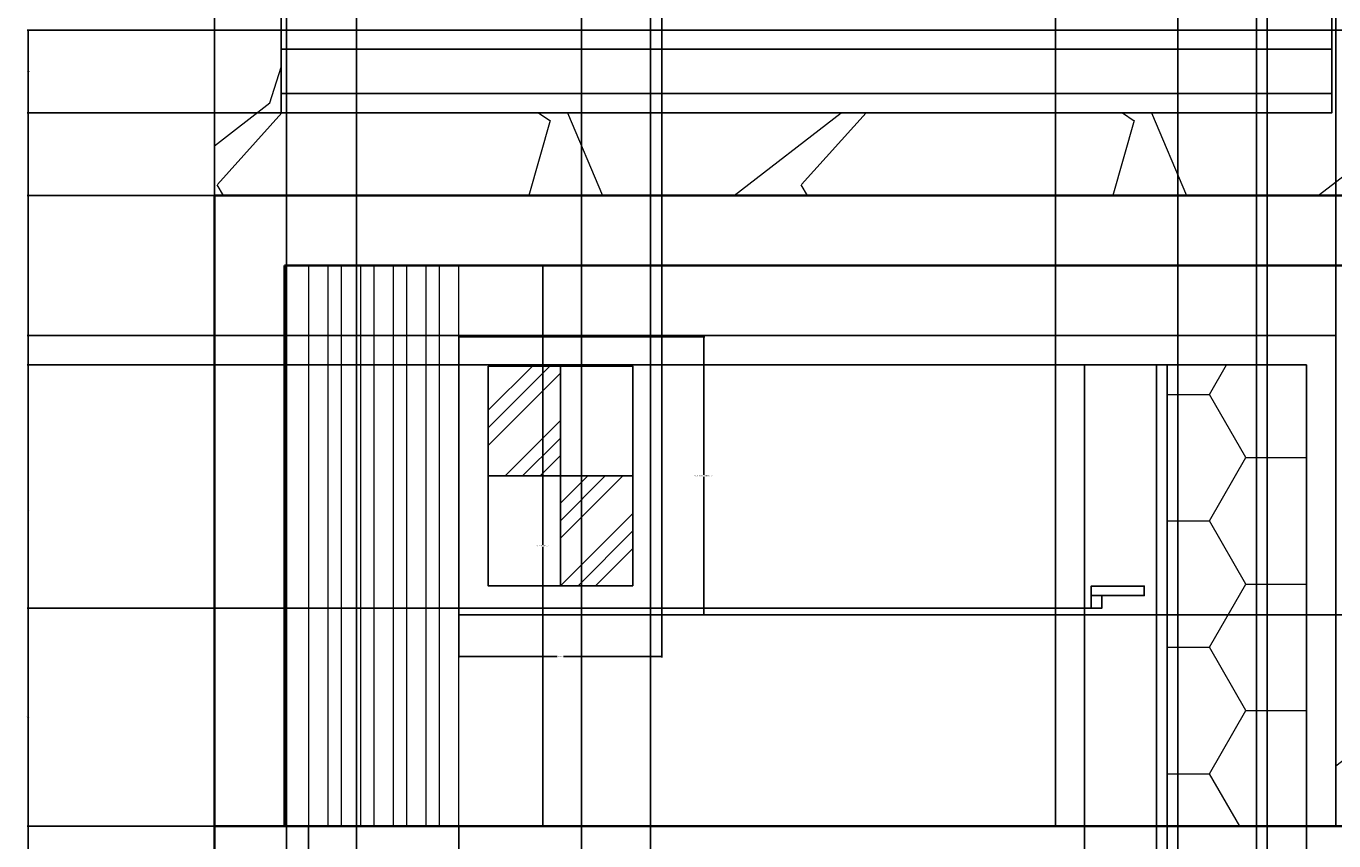
# Model space of a CAD drawing. Units: inches. Extents: x -8 to 554, y -200 to 499.
# Tile 7 of 12: x -8 to 216, y 233 to 372. Entities that reach past the tile are written whole.
import ezdxf

# ---------------------------------------------------------------- set-up
doc = ezdxf.new("R2010")
doc.units = ezdxf.units.IN
doc.header["$MEASUREMENT"] = 0
for name, color, linetype, lineweight in [('A-ANNO-DIMS', 2, 'Continuous', 18), ('A-DOOR', 3, 'Continuous', 25), ('A-DOOR-PATT', 252, 'Continuous', 13), ('A-FLOR', 7, 'Continuous', 35), ('A-GLAZ', 4, 'Continuous', 25), ('A-GLAZ-PATT', 252, 'Continuous', 13), ('A-WALL', 7, 'Continuous', 35), ('A-WALL-PATT', 252, 'Continuous', 13), ('A-WALL-PRPT', 7, 'Continuous', 25), ('A-WALL-SCRN', 8, 'Continuous', 18)]:
    doc.layers.add(name, color=color, linetype=linetype, lineweight=lineweight)
doc.styles.get("Standard").update_dxf_attribs({"font": 'arial.ttf'})
doc.dimstyles.get("Standard").update_dxf_attribs({"dimtxt": 0.18, "dimasz": 0.18, "dimexe": 0.18, "dimexo": 0.0625, "dimgap": 0.09, "dimtad": 0, "dimtih": 1, "dimtoh": 1, "dimdec": 4, "dimzin": 0, "dimdsep": 46, "dimtxsty": 'Standard', "dimcen": 0.09, "dimadec": 0, "dimazin": 0, "dimtfac": 1, "dimtdec": 4, "dimtofl": 0, "dimtmove": 0, "dimatfit": 3, "dimfxl": 1, "dimtolj": 1, "dimtzin": 0, "dimarcsym": 0})

# ---------------------------------------------------------------- blocks, each defined once
blk = doc.blocks.new('DOOR-LEVER-ELEV')
for points in [[(0, 2.19), (9.08, 2.19), (9.08, 3.81), (0, 3.81)], [(0, 2.19), (1.8, 2.19), (1.8, 0), (0, 0)]]:
    blk.add_lwpolyline(points, close=True)
blk = doc.blocks.new('SCREEN-FIVE-FINS-ELEV')
for points in [[(0, 0), (3.37, 0), (3.37, 96), (0, 96)], [(5.59, 0), (8.97, 0), (8.97, 96), (5.59, 96)], [(11.19, 0), (14.56, 0), (14.56, 96), (11.19, 96)], [(16.78, 0), (20.16, 0), (20.16, 96), (16.78, 96)], [(22.38, 0), (25.75, 0), (25.75, 96), (22.38, 96)]]:
    blk.add_lwpolyline(points, close=True)
blk = doc.blocks.new('WINDOW-CASING-FOUR-LIGHT')
blk.add_lwpolyline([(0, 47.61), (34.77, 47.61), (34.77, 0), (0, 0)], close=True)
blk = doc.blocks.new('*D18')
at = {"layer": 'A-ANNO-DIMS', "color": 0, "lineweight": -2, "transparency": 16777216}
for p, q in [((66.27, 331.48), (80.78, 331.48)), ((80.6, 331.3), (80.6, 283.66)), ((80.6, 235.66), (80.6, 283.3)), ((66.27, 235.48), (80.78, 235.48))]:
    blk.add_line(p, q, dxfattribs=at)
at = {"layer": 'A-ANNO-DIMS', "color": 0, "transparency": 16777216}
for points in [[(80.57, 331.3), (80.63, 331.3), (80.6, 331.48)], [(80.57, 235.66), (80.63, 235.66), (80.6, 235.48)]]:
    blk.add_solid(points, dxfattribs=at)
at = {"layer": 'Defpoints', "color": 0, "transparency": 16777216}
for p in [(66.2, 331.48), (80.6, 331.48), (66.2, 235.48)]:
    blk.add_point(p, dxfattribs=at)
at = {"layer": 'A-ANNO-DIMS', "color": 0, "transparency": 16777216, "insert": (80.6, 283.48), "char_height": 0.18, "attachment_point": 5}
blk.add_mtext('\\A1;FIN SCREEN 96 TYP.', dxfattribs=at)
blk = doc.blocks.new('*D19')
at = {"layer": 'A-ANNO-DIMS', "color": 0, "lineweight": -2, "transparency": 16777216}
for p, q in [((40.45, 235.42), (40.45, 220.9)), ((66.2, 235.42), (66.2, 220.9)), ((40.63, 221.08), (52.8, 221.08)), ((66.02, 221.08), (53.86, 221.08))]:
    blk.add_line(p, q, dxfattribs=at)
at = {"layer": 'A-ANNO-DIMS', "color": 0, "transparency": 16777216}
for points in [[(40.63, 221.11), (40.63, 221.05), (40.45, 221.08)], [(66.02, 221.11), (66.02, 221.05), (66.2, 221.08)]]:
    blk.add_solid(points, dxfattribs=at)
at = {"layer": 'Defpoints', "color": 0, "transparency": 16777216}
for p in [(40.45, 235.48), (66.2, 235.48), (66.2, 221.08)]:
    blk.add_point(p, dxfattribs=at)
at = {"layer": 'A-ANNO-DIMS', "color": 0, "transparency": 16777216, "insert": (53.33, 221.08), "char_height": 0.18, "attachment_point": 5}
blk.add_mtext('\\A1;26 TYP.', dxfattribs=at)
blk = doc.blocks.new('*D24')
at = {"layer": 'A-ANNO-DIMS', "color": 0, "lineweight": -2, "transparency": 16777216}
for p, q in [((101.04, 319.27), (108.3, 319.27)), ((108.12, 319.09), (108.12, 295.65)), ((108.12, 271.84), (108.12, 295.28)), ((101.04, 271.66), (108.3, 271.66))]:
    blk.add_line(p, q, dxfattribs=at)
at = {"layer": 'A-ANNO-DIMS', "color": 0, "transparency": 16777216}
for points in [[(108.09, 319.09), (108.15, 319.09), (108.12, 319.27)], [(108.09, 271.84), (108.15, 271.84), (108.12, 271.66)]]:
    blk.add_solid(points, dxfattribs=at)
at = {"layer": 'Defpoints', "color": 0, "transparency": 16777216}
for p in [(100.98, 319.27), (108.12, 319.27), (100.98, 271.66)]:
    blk.add_point(p, dxfattribs=at)
at = {"layer": 'A-ANNO-DIMS', "color": 0, "transparency": 16777216, "insert": (108.12, 295.47), "char_height": 0.18, "attachment_point": 5}
blk.add_mtext('\\A1;FOUR-LIGHT CASING 48 TYP.', dxfattribs=at)
blk = doc.blocks.new('*D25')
at = {"layer": 'A-ANNO-DIMS', "color": 0, "lineweight": -2, "transparency": 16777216}
for p, q in [((66.2, 271.6), (66.2, 264.34)), ((100.98, 271.6), (100.98, 264.34)), ((66.38, 264.52), (83.06, 264.52)), ((100.8, 264.52), (84.12, 264.52))]:
    blk.add_line(p, q, dxfattribs=at)
at = {"layer": 'A-ANNO-DIMS', "color": 0, "transparency": 16777216}
for points in [[(66.38, 264.55), (66.38, 264.49), (66.2, 264.52)], [(100.8, 264.55), (100.8, 264.49), (100.98, 264.52)]]:
    blk.add_solid(points, dxfattribs=at)
at = {"layer": 'Defpoints', "color": 0, "transparency": 16777216}
for p in [(66.2, 271.66), (100.98, 271.66), (100.98, 264.52)]:
    blk.add_point(p, dxfattribs=at)
at = {"layer": 'A-ANNO-DIMS', "color": 0, "transparency": 16777216, "insert": (83.59, 264.52), "char_height": 0.18, "attachment_point": 5}
blk.add_mtext('\\A1;35 TYP.', dxfattribs=at)
blk = doc.blocks.new('*D35')
at = {"layer": 'A-ANNO-DIMS', "color": 0, "lineweight": -2, "transparency": 16777216}
for p, q in [((24.28, 235.48), (-7.69, 235.48)), ((-7.51, 235.3), (-7.51, 181.66)), ((-7.51, 127.66), (-7.51, 181.3)), ((24.28, 127.48), (-7.69, 127.48))]:
    blk.add_line(p, q, dxfattribs=at)
at = {"layer": 'A-ANNO-DIMS', "color": 0, "transparency": 16777216}
for points in [[(-7.54, 235.3), (-7.48, 235.3), (-7.51, 235.48)], [(-7.54, 127.66), (-7.48, 127.66), (-7.51, 127.48)]]:
    blk.add_solid(points, dxfattribs=at)
at = {"layer": 'Defpoints', "color": 0, "transparency": 16777216}
for p in [(-7.51, 235.48), (24.34, 235.48), (24.34, 127.48)]:
    blk.add_point(p, dxfattribs=at)
at = {"layer": 'A-ANNO-DIMS', "color": 0, "transparency": 16777216, "insert": (-7.51, 181.48), "char_height": 0.18, "attachment_point": 5}
blk.add_mtext('\\A1;108', dxfattribs=at)
blk = doc.blocks.new('*D36')
at = {"layer": 'A-ANNO-DIMS', "color": 0, "lineweight": -2, "transparency": 16777216}
for p, q in [((24.28, 343.48), (-7.69, 343.48)), ((-7.51, 343.3), (-7.51, 289.66)), ((-7.51, 235.66), (-7.51, 289.3)), ((24.28, 235.48), (-7.69, 235.48))]:
    blk.add_line(p, q, dxfattribs=at)
at = {"layer": 'A-ANNO-DIMS', "color": 0, "transparency": 16777216}
for points in [[(-7.54, 343.3), (-7.48, 343.3), (-7.51, 343.48)], [(-7.54, 235.66), (-7.48, 235.66), (-7.51, 235.48)]]:
    blk.add_solid(points, dxfattribs=at)
at = {"layer": 'Defpoints', "color": 0, "transparency": 16777216}
for p in [(-7.51, 343.48), (24.34, 343.48), (24.34, 235.48)]:
    blk.add_point(p, dxfattribs=at)
at = {"layer": 'A-ANNO-DIMS', "color": 0, "transparency": 16777216, "insert": (-7.51, 289.48), "char_height": 0.18, "attachment_point": 5}
blk.add_mtext('\\A1;108', dxfattribs=at)
blk = doc.blocks.new('*D37')
at = {"layer": 'A-ANNO-DIMS', "color": 0, "lineweight": -2, "transparency": 16777216}
for p, q in [((24.28, 371.79), (-7.69, 371.79)), ((-7.51, 371.61), (-7.51, 357.82)), ((-7.51, 343.66), (-7.51, 357.45)), ((24.28, 343.48), (-7.69, 343.48))]:
    blk.add_line(p, q, dxfattribs=at)
at = {"layer": 'A-ANNO-DIMS', "color": 0, "transparency": 16777216}
for points in [[(-7.54, 371.61), (-7.48, 371.61), (-7.51, 371.79)], [(-7.54, 343.66), (-7.48, 343.66), (-7.51, 343.48)]]:
    blk.add_solid(points, dxfattribs=at)
at = {"layer": 'Defpoints', "color": 0, "transparency": 16777216}
for p in [(-7.51, 371.79), (24.34, 371.79), (24.34, 343.48)]:
    blk.add_point(p, dxfattribs=at)
at = {"layer": 'A-ANNO-DIMS', "color": 0, "transparency": 16777216, "insert": (-7.51, 357.64), "char_height": 0.18, "attachment_point": 5}
blk.add_mtext('\\A1;28.31', dxfattribs=at)
blk = doc.blocks.new('*D41')
at = {"layer": 'A-ANNO-DIMS', "color": 0, "lineweight": -2, "transparency": 16777216}
for p, q in [((24.34, 235.42), (24.34, -199.97)), ((40.45, 235.42), (40.45, -199.97)), ((24.52, -199.79), (31.94, -199.79)), ((40.27, -199.79), (32.85, -199.79))]:
    blk.add_line(p, q, dxfattribs=at)
at = {"layer": 'A-ANNO-DIMS', "color": 0, "transparency": 16777216}
for points in [[(24.52, -199.76), (24.52, -199.82), (24.34, -199.79)], [(40.27, -199.76), (40.27, -199.82), (40.45, -199.79)]]:
    blk.add_solid(points, dxfattribs=at)
at = {"layer": 'Defpoints', "color": 0, "transparency": 16777216}
for p in [(24.34, 235.48), (40.45, 235.48), (40.45, -199.79)]:
    blk.add_point(p, dxfattribs=at)
at = {"layer": 'A-ANNO-DIMS', "color": 0, "transparency": 16777216, "insert": (32.4, -199.79), "char_height": 0.18, "attachment_point": 5}
blk.add_mtext('\\A1;16.113', dxfattribs=at)
blk = doc.blocks.new('*D42')
at = {"layer": 'A-ANNO-DIMS', "color": 0, "lineweight": -2, "transparency": 16777216}
for p, q in [((100.98, 319.33), (100.98, 498.99)), ((101.16, 498.81), (134.27, 498.81)), ((168.16, 498.81), (135.05, 498.81)), ((168.34, 319.54), (168.34, 498.99))]:
    blk.add_line(p, q, dxfattribs=at)
at = {"layer": 'A-ANNO-DIMS', "color": 0, "transparency": 16777216}
for points in [[(101.16, 498.84), (101.16, 498.78), (100.98, 498.81)], [(168.16, 498.84), (168.16, 498.78), (168.34, 498.81)]]:
    blk.add_solid(points, dxfattribs=at)
at = {"layer": 'Defpoints', "color": 0, "transparency": 16777216}
for p in [(168.34, 498.81), (100.98, 319.27), (168.34, 319.48)]:
    blk.add_point(p, dxfattribs=at)
at = {"layer": 'A-ANNO-DIMS', "color": 0, "transparency": 16777216, "insert": (134.66, 498.81), "char_height": 0.18, "attachment_point": 5}
blk.add_mtext('\\A1;67.37', dxfattribs=at)
blk = doc.blocks.new('*D43')
at = {"layer": 'A-ANNO-DIMS', "color": 0, "lineweight": -2, "transparency": 16777216}
for p, q in [((168.34, 319.54), (168.34, 498.99)), ((168.52, 498.81), (192.12, 498.81)), ((216.16, 498.81), (192.56, 498.81)), ((216.34, 319.54), (216.34, 498.99))]:
    blk.add_line(p, q, dxfattribs=at)
at = {"layer": 'A-ANNO-DIMS', "color": 0, "transparency": 16777216}
for points in [[(168.52, 498.84), (168.52, 498.78), (168.34, 498.81)], [(216.16, 498.84), (216.16, 498.78), (216.34, 498.81)]]:
    blk.add_solid(points, dxfattribs=at)
at = {"layer": 'Defpoints', "color": 0, "transparency": 16777216}
for p in [(216.34, 498.81), (168.34, 319.48), (216.34, 319.48)]:
    blk.add_point(p, dxfattribs=at)
at = {"layer": 'A-ANNO-DIMS', "color": 0, "transparency": 16777216, "insert": (192.34, 498.81), "char_height": 0.18, "attachment_point": 5}
blk.add_mtext('\\A1;48', dxfattribs=at)
blk = doc.blocks.new('*D44')
at = {"layer": 'A-ANNO-DIMS', "color": 0, "lineweight": -2, "transparency": 16777216}
for p, q in [((168.28, 319.48), (-7.69, 319.48)), ((-7.51, 319.3), (-7.51, 277.66)), ((-7.51, 235.66), (-7.51, 277.3)), ((168.28, 235.48), (-7.69, 235.48))]:
    blk.add_line(p, q, dxfattribs=at)
at = {"layer": 'A-ANNO-DIMS', "color": 0, "transparency": 16777216}
for points in [[(-7.54, 319.3), (-7.48, 319.3), (-7.51, 319.48)], [(-7.54, 235.66), (-7.48, 235.66), (-7.51, 235.48)]]:
    blk.add_solid(points, dxfattribs=at)
at = {"layer": 'Defpoints', "color": 0, "transparency": 16777216}
for p in [(-7.51, 319.48), (168.34, 319.48), (168.34, 235.48)]:
    blk.add_point(p, dxfattribs=at)
at = {"layer": 'A-ANNO-DIMS', "color": 0, "transparency": 16777216, "insert": (-7.51, 277.48), "char_height": 0.18, "attachment_point": 5}
blk.add_mtext('\\A1;84', dxfattribs=at)
blk = doc.blocks.new('*D46')
at = {"layer": 'A-ANNO-DIMS', "color": 0, "lineweight": -2, "transparency": 16777216}
for p, q in [((101.04, 271.66), (554.26, 271.66)), ((554.08, 271.48), (554.08, 253.75)), ((554.08, 235.66), (554.08, 253.39)), ((66.27, 235.48), (554.26, 235.48))]:
    blk.add_line(p, q, dxfattribs=at)
at = {"layer": 'A-ANNO-DIMS', "color": 0, "transparency": 16777216}
for points in [[(554.05, 271.48), (554.11, 271.48), (554.08, 271.66)], [(554.05, 235.66), (554.11, 235.66), (554.08, 235.48)]]:
    blk.add_solid(points, dxfattribs=at)
at = {"layer": 'Defpoints', "color": 0, "transparency": 16777216}
for p in [(100.98, 271.66), (66.2, 235.48), (554.08, 235.48)]:
    blk.add_point(p, dxfattribs=at)
at = {"layer": 'A-ANNO-DIMS', "color": 0, "transparency": 16777216, "insert": (554.08, 253.57), "char_height": 0.18, "attachment_point": 5}
blk.add_mtext('\\A1;36.18', dxfattribs=at)
blk = doc.blocks.new('*D55')
at = {"layer": 'A-ANNO-DIMS', "color": 0, "lineweight": -2, "transparency": 16777216}
for p, q in [((204.61, -30.61), (204.61, 498.99)), ((204.79, 498.81), (328.57, 498.81)), ((453.14, 498.81), (329.36, 498.81)), ((453.32, -30.61), (453.32, 498.99))]:
    blk.add_line(p, q, dxfattribs=at)
at = {"layer": 'A-ANNO-DIMS', "color": 0, "transparency": 16777216}
for points in [[(204.79, 498.84), (204.79, 498.78), (204.61, 498.81)], [(453.14, 498.84), (453.14, 498.78), (453.32, 498.81)]]:
    blk.add_solid(points, dxfattribs=at)
at = {"layer": 'Defpoints', "color": 0, "transparency": 16777216}
for p in [(453.32, 498.81), (204.61, -30.67), (453.32, -30.67)]:
    blk.add_point(p, dxfattribs=at)
at = {"layer": 'A-ANNO-DIMS', "color": 0, "transparency": 16777216, "insert": (328.96, 498.81), "char_height": 0.18, "attachment_point": 5}
blk.add_mtext('\\A1;248.7', dxfattribs=at)
blk = doc.blocks.new('*D56')
at = {"layer": 'A-ANNO-DIMS', "color": 0, "lineweight": -2, "transparency": 16777216}
for p, q in [((24.34, 7.54), (24.34, 498.99)), ((24.52, 498.81), (30.06, 498.81)), ((36.51, 498.81), (30.97, 498.81)), ((36.69, 7.54), (36.69, 498.99))]:
    blk.add_line(p, q, dxfattribs=at)
at = {"layer": 'A-ANNO-DIMS', "color": 0, "transparency": 16777216}
for points in [[(24.52, 498.84), (24.52, 498.78), (24.34, 498.81)], [(36.51, 498.84), (36.51, 498.78), (36.69, 498.81)]]:
    blk.add_solid(points, dxfattribs=at)
at = {"layer": 'Defpoints', "color": 0, "transparency": 16777216}
for p in [(36.69, 498.81), (24.34, 7.48), (36.69, 7.48)]:
    blk.add_point(p, dxfattribs=at)
at = {"layer": 'A-ANNO-DIMS', "color": 0, "transparency": 16777216, "insert": (30.52, 498.81), "char_height": 0.18, "attachment_point": 5}
blk.add_mtext('\\A1;12.346', dxfattribs=at)
blk = doc.blocks.new('*D57')
at = {"layer": 'A-ANNO-DIMS', "color": 0, "lineweight": -2, "transparency": 16777216}
for p, q in [((36.69, -52.46), (36.69, 498.99)), ((36.87, 498.81), (42.48, 498.81)), ((48.51, 498.81), (42.9, 498.81)), ((48.69, -52.46), (48.69, 498.99))]:
    blk.add_line(p, q, dxfattribs=at)
at = {"layer": 'A-ANNO-DIMS', "color": 0, "transparency": 16777216}
for points in [[(36.87, 498.84), (36.87, 498.78), (36.69, 498.81)], [(48.51, 498.84), (48.51, 498.78), (48.69, 498.81)]]:
    blk.add_solid(points, dxfattribs=at)
at = {"layer": 'Defpoints', "color": 0, "transparency": 16777216}
for p in [(48.69, 498.81), (36.69, -52.52), (48.69, -52.52)]:
    blk.add_point(p, dxfattribs=at)
at = {"layer": 'A-ANNO-DIMS', "color": 0, "transparency": 16777216, "insert": (42.69, 498.81), "char_height": 0.18, "attachment_point": 5}
blk.add_mtext('\\A1;12', dxfattribs=at)
blk = doc.blocks.new('*D58')
at = {"layer": 'A-ANNO-DIMS', "color": 0, "lineweight": -2, "transparency": 16777216}
for p, q in [((36.69, 7.54), (36.69, 498.99)), ((36.87, 498.81), (61.56, 498.81)), ((87.03, 498.81), (62.34, 498.81)), ((87.21, 7.54), (87.21, 498.99))]:
    blk.add_line(p, q, dxfattribs=at)
at = {"layer": 'A-ANNO-DIMS', "color": 0, "transparency": 16777216}
for points in [[(36.87, 498.84), (36.87, 498.78), (36.69, 498.81)], [(87.03, 498.84), (87.03, 498.78), (87.21, 498.81)]]:
    blk.add_solid(points, dxfattribs=at)
at = {"layer": 'Defpoints', "color": 0, "transparency": 16777216}
for p in [(87.21, 498.81), (36.69, 7.48), (87.21, 7.48)]:
    blk.add_point(p, dxfattribs=at)
at = {"layer": 'A-ANNO-DIMS', "color": 0, "transparency": 16777216, "insert": (61.95, 498.81), "char_height": 0.18, "attachment_point": 5}
blk.add_mtext('\\A1;50.52', dxfattribs=at)
blk = doc.blocks.new('*D59')
at = {"layer": 'A-ANNO-DIMS', "color": 0, "lineweight": -2, "transparency": 16777216}
for p, q in [((87.21, -60.84), (87.21, 498.99)), ((87.39, 498.81), (92.67, 498.81)), ((98.86, 498.81), (93.58, 498.81)), ((99.04, -60.84), (99.04, 498.99))]:
    blk.add_line(p, q, dxfattribs=at)
at = {"layer": 'A-ANNO-DIMS', "color": 0, "transparency": 16777216}
for points in [[(87.39, 498.84), (87.39, 498.78), (87.21, 498.81)], [(98.86, 498.84), (98.86, 498.78), (99.04, 498.81)]]:
    blk.add_solid(points, dxfattribs=at)
at = {"layer": 'Defpoints', "color": 0, "transparency": 16777216}
for p in [(99.04, 498.81), (87.21, -60.9), (99.04, -60.9)]:
    blk.add_point(p, dxfattribs=at)
at = {"layer": 'A-ANNO-DIMS', "color": 0, "transparency": 16777216, "insert": (93.12, 498.81), "char_height": 0.18, "attachment_point": 5}
blk.add_mtext('\\A1;11.827', dxfattribs=at)
blk = doc.blocks.new('*D60')
at = {"layer": 'A-ANNO-DIMS', "color": 0, "lineweight": -2, "transparency": 16777216}
for p, q in [((87.21, 7.54), (87.21, 498.99)), ((87.39, 498.81), (137.89, 498.81)), ((189.12, 498.81), (138.63, 498.81)), ((189.3, 7.54), (189.3, 498.99))]:
    blk.add_line(p, q, dxfattribs=at)
at = {"layer": 'A-ANNO-DIMS', "color": 0, "transparency": 16777216}
for points in [[(87.39, 498.84), (87.39, 498.78), (87.21, 498.81)], [(189.12, 498.84), (189.12, 498.78), (189.3, 498.81)]]:
    blk.add_solid(points, dxfattribs=at)
at = {"layer": 'Defpoints', "color": 0, "transparency": 16777216}
for p in [(189.3, 498.81), (87.21, 7.48), (189.3, 7.48)]:
    blk.add_point(p, dxfattribs=at)
at = {"layer": 'A-ANNO-DIMS', "color": 0, "transparency": 16777216, "insert": (138.26, 498.81), "char_height": 0.18, "attachment_point": 5}
blk.add_mtext('\\A1;102.1', dxfattribs=at)
blk = doc.blocks.new('*D61')
at = {"layer": 'A-ANNO-DIMS', "color": 0, "lineweight": -2, "transparency": 16777216}
for p, q in [((189.3, -52.46), (189.3, 498.99)), ((189.48, 498.81), (195.57, 498.81)), ((202.57, 498.81), (196.48, 498.81)), ((202.75, -52.46), (202.75, 498.99))]:
    blk.add_line(p, q, dxfattribs=at)
at = {"layer": 'A-ANNO-DIMS', "color": 0, "transparency": 16777216}
for points in [[(189.48, 498.84), (189.48, 498.78), (189.3, 498.81)], [(202.57, 498.84), (202.57, 498.78), (202.75, 498.81)]]:
    blk.add_solid(points, dxfattribs=at)
at = {"layer": 'Defpoints', "color": 0, "transparency": 16777216}
for p in [(202.75, 498.81), (189.3, -52.52), (202.75, -52.52)]:
    blk.add_point(p, dxfattribs=at)
at = {"layer": 'A-ANNO-DIMS', "color": 0, "transparency": 16777216, "insert": (196.03, 498.81), "char_height": 0.18, "attachment_point": 5}
blk.add_mtext('\\A1;13.446', dxfattribs=at)
blk = doc.blocks.new('*D62')
at = {"layer": 'A-ANNO-DIMS', "color": 0, "lineweight": -2, "transparency": 16777216}
for p, q in [((189.3, 7.54), (189.3, 498.99)), ((189.48, 498.81), (263.01, 498.81)), ((337.31, 498.81), (263.78, 498.81)), ((337.49, 7.54), (337.49, 498.99))]:
    blk.add_line(p, q, dxfattribs=at)
at = {"layer": 'A-ANNO-DIMS', "color": 0, "transparency": 16777216}
for points in [[(189.48, 498.84), (189.48, 498.78), (189.3, 498.81)], [(337.31, 498.84), (337.31, 498.78), (337.49, 498.81)]]:
    blk.add_solid(points, dxfattribs=at)
at = {"layer": 'Defpoints', "color": 0, "transparency": 16777216}
for p in [(337.49, 498.81), (189.3, 7.48), (337.49, 7.48)]:
    blk.add_point(p, dxfattribs=at)
at = {"layer": 'A-ANNO-DIMS', "color": 0, "transparency": 16777216, "insert": (263.4, 498.81), "char_height": 0.18, "attachment_point": 5}
blk.add_mtext('\\A1;148.2', dxfattribs=at)
blk = doc.blocks.new('*D70')
at = {"layer": 'A-ANNO-DIMS', "color": 0, "lineweight": -2, "transparency": 16777216}
for p, q in [((35.79, 357.7), (35.79, 498.99)), ((35.97, 498.81), (125.35, 498.81)), ((215.5, 498.81), (126.12, 498.81)), ((215.68, 357.7), (215.68, 498.99))]:
    blk.add_line(p, q, dxfattribs=at)
at = {"layer": 'A-ANNO-DIMS', "color": 0, "transparency": 16777216}
for points in [[(35.97, 498.84), (35.97, 498.78), (35.79, 498.81)], [(215.5, 498.84), (215.5, 498.78), (215.68, 498.81)]]:
    blk.add_solid(points, dxfattribs=at)
at = {"layer": 'Defpoints', "color": 0, "transparency": 16777216}
for p in [(215.68, 498.81), (35.79, 357.64), (215.68, 357.64)]:
    blk.add_point(p, dxfattribs=at)
at = {"layer": 'A-ANNO-DIMS', "color": 0, "transparency": 16777216, "insert": (125.73, 498.81), "char_height": 0.18, "attachment_point": 5}
blk.add_mtext('\\A1;179.9', dxfattribs=at)
blk = doc.blocks.new('*D72')
at = {"layer": 'A-ANNO-DIMS', "color": 0, "lineweight": -2, "transparency": 16777216}
for p, q in [((24.34, 371.85), (24.34, 498.99)), ((24.52, 498.81), (29.61, 498.81)), ((35.61, 498.81), (30.52, 498.81)), ((35.79, 371.85), (35.79, 498.99))]:
    blk.add_line(p, q, dxfattribs=at)
at = {"layer": 'A-ANNO-DIMS', "color": 0, "transparency": 16777216}
for points in [[(24.52, 498.84), (24.52, 498.78), (24.34, 498.81)], [(35.61, 498.84), (35.61, 498.78), (35.79, 498.81)]]:
    blk.add_solid(points, dxfattribs=at)
at = {"layer": 'Defpoints', "color": 0, "transparency": 16777216}
for p in [(35.79, 498.81), (24.34, 371.79), (35.79, 371.79)]:
    blk.add_point(p, dxfattribs=at)
at = {"layer": 'A-ANNO-DIMS', "color": 0, "transparency": 16777216, "insert": (30.06, 498.81), "char_height": 0.18, "attachment_point": 5}
blk.add_mtext('\\A1;11.445', dxfattribs=at)
blk = doc.blocks.new('*D73')
at = {"layer": 'A-ANNO-DIMS', "color": 0, "lineweight": -2, "transparency": 16777216}
for p, q in [((35.72, 371.79), (-7.69, 371.79)), ((-7.51, 371.61), (-7.51, 364.9)), ((-7.51, 357.82), (-7.51, 364.53)), ((35.72, 357.64), (-7.69, 357.64))]:
    blk.add_line(p, q, dxfattribs=at)
at = {"layer": 'A-ANNO-DIMS', "color": 0, "transparency": 16777216}
for points in [[(-7.54, 371.61), (-7.48, 371.61), (-7.51, 371.79)], [(-7.54, 357.82), (-7.48, 357.82), (-7.51, 357.64)]]:
    blk.add_solid(points, dxfattribs=at)
at = {"layer": 'Defpoints', "color": 0, "transparency": 16777216}
for p in [(-7.51, 371.79), (35.79, 371.79), (35.79, 357.64)]:
    blk.add_point(p, dxfattribs=at)
at = {"layer": 'A-ANNO-DIMS', "color": 0, "transparency": 16777216, "insert": (-7.51, 364.71), "char_height": 0.18, "attachment_point": 5}
blk.add_mtext('\\A1;14.155', dxfattribs=at)
blk = doc.blocks.new('*D80')
at = {"layer": 'A-ANNO-DIMS', "color": 0, "lineweight": -2, "transparency": 16777216}
for p, q in [((173.34, 314.42), (173.34, -199.97)), ((211.34, 314.42), (211.34, -199.97)), ((173.52, -199.79), (192.12, -199.79)), ((211.16, -199.79), (192.56, -199.79))]:
    blk.add_line(p, q, dxfattribs=at)
at = {"layer": 'A-ANNO-DIMS', "color": 0, "transparency": 16777216}
for points in [[(173.52, -199.76), (173.52, -199.82), (173.34, -199.79)], [(211.16, -199.76), (211.16, -199.82), (211.34, -199.79)]]:
    blk.add_solid(points, dxfattribs=at)
at = {"layer": 'Defpoints', "color": 0, "transparency": 16777216}
for p in [(173.34, 314.48), (211.34, 314.48), (211.34, -199.79)]:
    blk.add_point(p, dxfattribs=at)
at = {"layer": 'A-ANNO-DIMS', "color": 0, "transparency": 16777216, "insert": (192.34, -199.79), "char_height": 0.18, "attachment_point": 5}
blk.add_mtext('\\A1;38', dxfattribs=at)
blk = doc.blocks.new('*D81')
at = {"layer": 'A-ANNO-DIMS', "color": 0, "lineweight": -2, "transparency": 16777216}
for p, q in [((173.34, 235.42), (173.34, -199.97)), ((185.64, 235.42), (185.64, -199.97)), ((173.52, -199.79), (179.04, -199.79)), ((185.46, -199.79), (179.95, -199.79))]:
    blk.add_line(p, q, dxfattribs=at)
at = {"layer": 'A-ANNO-DIMS', "color": 0, "transparency": 16777216}
for points in [[(173.52, -199.76), (173.52, -199.82), (173.34, -199.79)], [(185.46, -199.76), (185.46, -199.82), (185.64, -199.79)]]:
    blk.add_solid(points, dxfattribs=at)
at = {"layer": 'Defpoints', "color": 0, "transparency": 16777216}
for p in [(173.34, 235.48), (185.64, 235.48), (185.64, -199.79)]:
    blk.add_point(p, dxfattribs=at)
at = {"layer": 'A-ANNO-DIMS', "color": 0, "transparency": 16777216, "insert": (179.49, -199.79), "char_height": 0.18, "attachment_point": 5}
blk.add_mtext('\\A1;12.302', dxfattribs=at)
blk = doc.blocks.new('*D82')
at = {"layer": 'A-ANNO-DIMS', "color": 0, "lineweight": -2, "transparency": 16777216}
for p, q in [((185.64, 235.42), (185.64, -199.97)), ((187.48, 235.42), (187.48, -199.97)), ((185.82, -199.79), (186.18, -199.79)), ((187.3, -199.79), (186.95, -199.79))]:
    blk.add_line(p, q, dxfattribs=at)
at = {"layer": 'A-ANNO-DIMS', "color": 0, "transparency": 16777216}
for points in [[(185.82, -199.76), (185.82, -199.82), (185.64, -199.79)], [(187.3, -199.76), (187.3, -199.82), (187.48, -199.79)]]:
    blk.add_solid(points, dxfattribs=at)
at = {"layer": 'Defpoints', "color": 0, "transparency": 16777216}
for p in [(185.64, 235.48), (187.48, 235.48), (187.48, -199.79)]:
    blk.add_point(p, dxfattribs=at)
at = {"layer": 'A-ANNO-DIMS', "color": 0, "transparency": 16777216, "insert": (186.56, -199.79), "char_height": 0.18, "attachment_point": 5}
blk.add_mtext('\\A1;1.837', dxfattribs=at)
blk = doc.blocks.new('*D83')
at = {"layer": 'A-ANNO-DIMS', "color": 0, "lineweight": -2, "transparency": 16777216}
for p, q in [((168.28, 319.48), (-7.69, 319.48)), ((-7.51, 319.3), (-7.51, 317.16)), ((-7.51, 314.66), (-7.51, 316.8)), ((173.28, 314.48), (-7.69, 314.48))]:
    blk.add_line(p, q, dxfattribs=at)
at = {"layer": 'A-ANNO-DIMS', "color": 0, "transparency": 16777216}
for points in [[(-7.54, 319.3), (-7.48, 319.3), (-7.51, 319.48)], [(-7.54, 314.66), (-7.48, 314.66), (-7.51, 314.48)]]:
    blk.add_solid(points, dxfattribs=at)
at = {"layer": 'Defpoints', "color": 0, "transparency": 16777216}
for p in [(-7.51, 319.48), (168.34, 319.48), (173.34, 314.48)]:
    blk.add_point(p, dxfattribs=at)
at = {"layer": 'A-ANNO-DIMS', "color": 0, "transparency": 16777216, "insert": (-7.51, 316.98), "char_height": 0.18, "attachment_point": 5}
blk.add_mtext('\\A1;5', dxfattribs=at)
blk = doc.blocks.new('*D84')
at = {"layer": 'A-ANNO-DIMS', "color": 0, "lineweight": -2, "transparency": 16777216}
for p, q in [((174.41, 272.79), (-7.69, 272.79)), ((-7.51, 272.61), (-7.51, 254.32)), ((-7.51, 235.66), (-7.51, 253.95)), ((173.28, 235.48), (-7.69, 235.48))]:
    blk.add_line(p, q, dxfattribs=at)
at = {"layer": 'A-ANNO-DIMS', "color": 0, "transparency": 16777216}
for points in [[(-7.54, 272.61), (-7.48, 272.61), (-7.51, 272.79)], [(-7.54, 235.66), (-7.48, 235.66), (-7.51, 235.48)]]:
    blk.add_solid(points, dxfattribs=at)
at = {"layer": 'Defpoints', "color": 0, "transparency": 16777216}
for p in [(174.48, 272.79), (-7.51, 235.48), (173.34, 235.48)]:
    blk.add_point(p, dxfattribs=at)
at = {"layer": 'A-ANNO-DIMS', "color": 0, "transparency": 16777216, "insert": (-7.51, 254.13), "char_height": 0.18, "attachment_point": 5}
blk.add_mtext('\\A1;37.31', dxfattribs=at)

msp = doc.modelspace()

# ---------------------------------------------------------------- hatches: boundary and pattern name
at = {"layer": 'A-DOOR-PATT', "transparency": 33554523}
h = msp.add_hatch(dxfattribs=at)
h.set_pattern_fill('HONEY', color=256, scale=100)
h.set_pattern_definition([(0, (-117.809, -80.312), (18.75, 10.82532), [12.5, -25]), (120, (-117.809, -80.312), (-18.75, 10.82532), [12.5, -25]), (60, (-117.809, -80.312), (4e-15, 21.65064), [-25, 12.5])])
h.paths.add_polyline_path([(211.3421, 314.4814), (187.4809, 314.4814), (187.4809, 235.4814), (211.3421, 235.4814)])
h.paths.add_polyline_path([(211.3421, 206.4814), (187.4809, 206.4814), (187.4809, 127.4814), (211.3421, 127.4814)])
h.paths.add_polyline_path([(211.3421, 98.4814), (187.4809, 98.4814), (187.4809, 19.4814), (211.3421, 19.4814)])
h.paths.add_polyline_path([(432.5174, 98.4814), (408.6562, 98.4814), (408.6562, 19.4814), (432.5174, 19.4814)])
h.paths.add_polyline_path([(432.5174, 206.4814), (408.6562, 206.4814), (408.6562, 127.4814), (432.5174, 127.4814), (432.5174, 155.7921)])
h.paths.add_polyline_path([(432.5174, 314.4814), (408.6562, 314.4814), (408.6562, 235.4814), (432.5174, 235.4814)])
at = {"layer": 'A-GLAZ-PATT'}
h = msp.add_hatch(dxfattribs=at)
h.set_pattern_fill('GOST_GROUND', color=256)
h.set_pattern_definition([(45, (-117.809, -80.312), (14.14214, 0), [20]), (45, (-114.809, -80.312), (14.14214, 0), [20]), (45, (-111.809, -80.312), (14.14214, 0), [20])])
h.paths.add_polyline_path([(83.5906, 206.2713), (71.2048, 206.2713), (71.2048, 187.4661), (83.5906, 187.4661)])
h.paths.add_polyline_path([(95.9765, 187.4661), (83.5906, 187.4661), (83.5906, 168.661), (95.9765, 168.661)])
h.paths.add_polyline_path([(83.5906, 98.2713), (71.2048, 98.2713), (71.2048, 79.4661), (83.5906, 79.4661)])
h.paths.add_polyline_path([(95.9765, 79.4661), (83.5906, 79.4661), (83.5906, 60.661), (95.9765, 60.661)])
h.paths.add_polyline_path([(333.2924, 98.788), (317.3421, 98.788), (317.3421, 61.7623), (333.2924, 61.7623)])
h.paths.add_polyline_path([(352.699, 98.788), (336.6386, 98.788), (336.6386, 61.7623), (352.699, 61.7623)])
h.paths.add_polyline_path([(333.2924, 206.788), (317.3421, 206.788), (317.3421, 169.7623), (333.2924, 169.7623)])
h.paths.add_polyline_path([(352.699, 206.788), (336.6386, 206.788), (336.6386, 169.7623), (352.699, 169.7623)])
h.paths.add_polyline_path([(333.2924, 314.788), (317.3421, 314.788), (317.3421, 277.7623), (333.2924, 277.7623)])
h.paths.add_polyline_path([(352.699, 314.788), (336.6386, 314.788), (336.6386, 277.7623), (352.699, 277.7623)])
h.paths.add_polyline_path([(95.9765, 295.4661), (83.5906, 295.4661), (83.5906, 276.661), (95.9765, 276.661)])
h.paths.add_polyline_path([(83.5906, 314.2713), (71.2048, 314.2713), (71.2048, 295.4661), (83.5906, 295.4661)])
at = {"layer": 'A-WALL-PATT'}
h = msp.add_hatch(dxfattribs=at)
h.set_pattern_fill('GRAVEL', color=256, scale=100)
h.set_pattern_definition([(228.0128, (-45.809, 19.688), (-800, -900), [13.4536, -1331.909]), (184.9697, (-54.8087, 9.688), (1200, 100), [23.0868, -2285.5925]), (132.5104, (-77.809, 7.688), (1000, -1100), [16.279, -1611.6033]), (267.2737, (-116.8087, -17.312), (100, 2000), [21.0238, -2081.3558]), (292.83365, (-117.8087, -38.312), (-500, 1200), [20.6155, -2040.9373]), (357.2737, (-109.8087, -57.312), (-2000, 100), [21.0238, -2081.3558]), (37.69424, (-88.8087, -58.3118), (-1300, -1000), [27.803, -2752.4849]), (72.2553, (-66.8087, -41.312), (700, 2200), [26.2488, -2598.632]), (121.4296, (-58.8087, -16.312), (-800, 1300), [21.095, -2088.4073]), (175.2364, (-69.809, 1.688), (1100, -100), [24.083, -1180.076]), (222.39744, (-93.8087, 3.6882), (-1200, -1100), [31.1448, -3083.3375]), (138.814, (-17.809, -18.312), (-700, 600), [10.63, -1052.3845]), (171.4692, (-25.8087, -11.312), (1300, -200), [20.2237, -2002.151]), (225, (-45.81, -8.31), (-1e-14, -100), [14.142, -127.279]), (203.1986, (-52.809, 3.688), (500, 200), [7.616, -753.9615]), (291.8014, (-59.809, 0.688), (-100, 300), [10.77, -527.746]), (30.9638, (-55.809, -9.312), (300, 200), [17.493, -565.602]), (161.565, (-40.81, -0.312), (200, -100), [12.649, -303.579]), (16.3895, (-117.8087, 0.688), (1000, 300), [17.72, -1754.2845]), (70.3462, (-100.809, 5.688), (-400, -1100), [14.866, -1471.741]), (293.1986, (-40.809, 19.688), (-200, 500), [15.2315, -746.346]), (343.6105, (-34.8087, 5.688), (-1000, 300), [17.72, -1754.2845]), (339.444, (-117.809, -61.312), (-500, 200), [17.088, -837.3124]), (294.7751, (-101.809, -67.312), (-500, 1100), [14.318, -1417.4643]), (66.8014, (-39.809, -80.312), (200, 500), [15.2315, -746.346]), (17.354, (-33.809, -66.312), (-1300, -400), [16.763, -1659.5424]), (69.444, (-88.809, -80.312), (-200, -500), [8.544, -845.8564]), (101.31, (-45.809, -80.312), (-100, 400), [5.099, -504.803]), (165.9638, (-46.809, -75.312), (300, -100), [20.6155, -391.695]), (186.009, (-66.8087, -70.312), (1000, 100), [19.105, -1891.3923]), (303.69, (-55.81, -18.312), (-100, 200), [14.422, -346.133]), (353.1572, (-47.8087, -30.312), (1700, -200), [25.1794, -2492.7563]), (60.9454, (-22.809, -33.312), (-400, -700), [10.2956, -1019.2674]), (90, (-17.81, -24.31), (-100, 100), [6, -94]), (120.2564, (-68.809, -67.312), (400, -700), [13.8924, -1375.352]), (48.0128, (-75.809, -55.312), (800, 900), [26.907, -1318.455]), (0, (-57.81, -35.31), (100, 100), [26, -74]), (325.3048, (-31.809, -35.312), (1000, -700), [15.8114, -1565.3274]), (254.0546, (-18.809, -44.312), (-100, -400), [14.56, -713.451]), (207.646, (-22.8087, -58.312), (-1900, -1000), [23.7065, -2346.9474]), (175.4261, (-43.8087, -69.312), (-1300, 100), [25.08, -2482.9073])])
h.paths.add_polyline_path([(48.6882, -52.5186), (24.3421, -52.5186), (24.3421, -112.5186), (48.6882, -112.5186)])
h.paths.add_polyline_path([(212.2282, -52.5186), (140.2282, -52.5186), (128.2282, -52.5186), (128.2282, -112.5186), (140.2282, -112.5186), (140.2282, -64.9665), (202.9211, -64.9665), (202.9211, -112.5186), (212.2282, -112.5186)])
h.paths.add_polyline_path([(312.3421, 49.7921), (216.3421, 49.7921), (216.3421, 19.4814), (312.3421, 19.4814)])
h.paths.add_polyline_path([(312.3421, 157.7921), (216.3421, 157.7921), (216.3421, 127.4814), (312.3421, 127.4814)])
h.paths.add_polyline_path([(312.3421, 265.7921), (216.3421, 265.7921), (216.3421, 235.4814), (312.3421, 235.4814)])
h.paths.add_polyline_path([(432.5174, 371.7921), (215.6778, 371.7921), (215.6778, 368.5162), (215.6778, 357.6367), (35.7874, 357.6367), (35.7874, 360.9127), (35.7874, 371.7921), (24.3421, 371.7921), (24.3421, 343.4814), (35.7874, 343.4814), (432.5174, 343.4814)])

# ---------------------------------------------------------------- linework, layer by layer
at = {"layer": 'A-DOOR'}
for p, q in [((173.3421, 235.4814), (173.3421, 314.4814)), ((173.3421, 314.4814), (211.3421, 314.4814)), ((211.3421, 314.4814), (211.3421, 235.4814))]:
    msp.add_line(p, q, dxfattribs=at)
for points in [[(216.3421, 235.4814), (168.3421, 235.4814), (168.3421, 319.4814), (216.3421, 319.4814)], [(185.644, 314.4814), (187.4809, 314.4814), (187.4809, 235.4814), (185.644, 235.4814)]]:
    msp.add_lwpolyline(points, close=True, dxfattribs=at)
at = {"layer": 'A-FLOR'}
for p, q in [((432.5174, 343.4814), (24.3421, 343.4814)), ((444.3421, 331.4814), (36.3421, 331.4814)), ((444.3421, 235.4814), (24.3421, 235.4814)), ((36.3421, 235.4814), (444.3421, 235.4814))]:
    msp.add_line(p, q, dxfattribs=at)
at = {"layer": 'A-GLAZ'}
for p, q in [((83.5906, 314.2713), (83.5906, 276.661)), ((71.2048, 295.4661), (95.9765, 295.4661))]:
    msp.add_line(p, q, dxfattribs=at)
msp.add_lwpolyline([(71.2048, 314.2713), (95.9765, 314.2713), (95.9765, 276.661), (71.2048, 276.661)], close=True, dxfattribs=at)
at = {"layer": 'A-WALL'}
for p, q in [((24.3421, 343.4814), (24.3421, 223.4814)), ((36.3421, 331.4814), (36.3421, 235.4814)), ((24.3421, 235.4814), (24.3421, 115.4814))]:
    msp.add_line(p, q, dxfattribs=at)
at = {"layer": 'A-WALL-PRPT'}
for p, q in [((432.5174, 371.7921), (215.6778, 371.7921)), ((215.6778, 371.7921), (215.6778, 357.6367))]:
    msp.add_line(p, q, dxfattribs=at)
msp.add_lwpolyline([(35.7874, 357.6367), (35.7874, 371.7921), (24.3421, 371.7921), (24.3421, 343.4814), (35.7874, 343.4814)], dxfattribs=at)
for points in [[(35.7874, 371.7921), (215.6778, 371.7921), (215.6778, 368.5162), (35.7874, 368.5162)], [(35.7874, 360.9127), (215.6778, 360.9127), (215.6778, 357.6367), (35.7874, 357.6367)]]:
    msp.add_lwpolyline(points, close=True, dxfattribs=at)

# ---------------------------------------------------------------- block references
at = {"layer": 'A-DOOR'}
msp.add_blockref('DOOR-LEVER-ELEV', (174.4762, 272.7884), dxfattribs=at)
at = {"layer": 'A-GLAZ'}
msp.add_blockref('WINDOW-CASING-FOUR-LIGHT', (66.2048, 271.661), dxfattribs=at)
at = {"layer": 'A-WALL-SCRN'}
msp.add_blockref('SCREEN-FIVE-FINS-ELEV', (40.4549, 235.4814), dxfattribs=at)

# ---------------------------------------------------------------- dimensions: what is measured, and where the dimension line sits
at = {"layer": 'A-ANNO-DIMS'}
for base, p1, p2, override, picture, middle in [((36.6882, 498.8091), (24.3421, 7.4814), (36.6882, 7.4814), {"dimdec": 3, "dimlfac": 1, "dimrnd": 0, "dimzin": 0, "dimdsep": 46, "dimlunit": 2}, '*D56', (30.5151, 498.8091)), ((35.7874, 498.8091), (24.3421, 371.7921), (35.7874, 371.7921), {"dimdec": 3, "dimlfac": 1, "dimrnd": 0, "dimzin": 0, "dimdsep": 46, "dimlunit": 2}, '*D72', (30.0647, 498.8091)), ((215.6778, 498.8091), (35.7874, 357.6367), (215.6778, 357.6367), {"dimdec": 1, "dimlfac": 1, "dimrnd": 0, "dimzin": 0, "dimdsep": 46, "dimlunit": 2}, '*D70', (125.7326, 498.8091)), ((48.6882, 498.8091), (36.6882, -52.5186), (48.6882, -52.5186), {"dimdec": 0, "dimlfac": 1, "dimrnd": 0, "dimzin": 0, "dimdsep": 46, "dimlunit": 2}, '*D57', (42.6882, 498.8091)), ((87.21, 498.8091), (36.6882, 7.4814), (87.21, 7.4814), {"dimdec": 2, "dimlfac": 1, "dimrnd": 0, "dimzin": 0, "dimdsep": 46, "dimlunit": 2}, '*D58', (61.9491, 498.8091)), ((99.037, 498.8091), (87.21, -60.9032), (99.037, -60.9032), {"dimdec": 3, "dimlfac": 1, "dimrnd": 0, "dimzin": 0, "dimdsep": 46, "dimlunit": 2}, '*D59', (93.1235, 498.8091)), ((189.3049, 498.8091), (87.21, 7.4814), (189.3049, 7.4814), {"dimdec": 1, "dimlfac": 1, "dimrnd": 0, "dimzin": 0, "dimdsep": 46, "dimlunit": 2}, '*D60', (138.2575, 498.8091)), ((168.3421, 498.8091), (100.9765, 319.2713), (168.3421, 319.4814), {"dimdec": 2, "dimlfac": 1, "dimrnd": 0, "dimzin": 0, "dimdsep": 46, "dimlunit": 2}, '*D42', (134.6593, 498.8091)), ((216.3421, 498.8091), (168.3421, 319.4814), (216.3421, 319.4814), {"dimdec": 0, "dimlfac": 1, "dimrnd": 0, "dimzin": 0, "dimdsep": 46, "dimlunit": 2}, '*D43', (192.3421, 498.8091)), ((202.7513, 498.8091), (189.3049, -52.5186), (202.7513, -52.5186), {"dimdec": 3, "dimlfac": 1, "dimrnd": 0, "dimzin": 0, "dimdsep": 46, "dimlunit": 2}, '*D61', (196.0281, 498.8091)), ((337.4923, 498.8091), (189.3049, 7.4814), (337.4923, 7.4814), {"dimdec": 1, "dimlfac": 1, "dimrnd": 0, "dimzin": 0, "dimdsep": 46, "dimlunit": 2}, '*D62', (263.3986, 498.8091)), ((453.3222, 498.8091), (204.6055, -30.6677), (453.3222, -30.6677), {"dimdec": 1, "dimlfac": 1, "dimrnd": 0, "dimzin": 0, "dimdsep": 46, "dimlunit": 2}, '*D55', (328.9639, 498.8091)), ((211.3421, -199.7912), (173.3421, 314.4814), (211.3421, 314.4814), {"dimdec": 0, "dimlfac": 1, "dimrnd": 0, "dimzin": 0, "dimdsep": 46, "dimlunit": 2}, '*D80', (192.3421, -199.7912)), ((40.4549, -199.7912), (24.3421, 235.4814), (40.4549, 235.4814), {"dimdec": 3, "dimlfac": 1, "dimrnd": 0, "dimzin": 0, "dimdsep": 46, "dimlunit": 2}, '*D41', (32.3985, -199.7912)), ((185.644, -199.7912), (173.3421, 235.4814), (185.644, 235.4814), {"dimdec": 3, "dimlfac": 1, "dimrnd": 0, "dimzin": 0, "dimdsep": 46, "dimlunit": 2}, '*D81', (179.493, -199.7912)), ((187.4809, -199.7912), (185.644, 235.4814), (187.4809, 235.4814), {"dimdec": 3, "dimlfac": 1, "dimrnd": 0, "dimzin": 0, "dimdsep": 46, "dimlunit": 2}, '*D82', (186.5625, -199.7912))]:
    dim = msp.add_linear_dim(base=base, p1=p1, p2=p2, dimstyle='Standard', override=override, dxfattribs=at)
    dim.commit()
    dim.dimension.update_dxf_attribs({"geometry": picture, "text_midpoint": middle})
for base, p1, p2, override, picture, middle in [((-7.5079, 371.7921), (35.7874, 357.6367), (35.7874, 371.7921), {"dimdec": 3, "dimlfac": 1, "dimrnd": 0, "dimzin": 0, "dimdsep": 46, "dimlunit": 2}, '*D73', (-7.5079, 364.7144)), ((-7.5079, 371.7921), (24.3421, 343.4814), (24.3421, 371.7921), {"dimdec": 2, "dimlfac": 1, "dimrnd": 0, "dimzin": 0, "dimdsep": 46, "dimlunit": 2}, '*D37', (-7.5079, 357.6367)), ((-7.5079, 343.4814), (24.3421, 235.4814), (24.3421, 343.4814), {"dimdec": 0, "dimlfac": 1, "dimrnd": 0, "dimzin": 0, "dimdsep": 46, "dimlunit": 2}, '*D36', (-7.5079, 289.4814)), ((-7.5079, 319.4814), (168.3421, 235.4814), (168.3421, 319.4814), {"dimdec": 0, "dimlfac": 1, "dimrnd": 0, "dimzin": 0, "dimdsep": 46, "dimlunit": 2}, '*D44', (-7.5079, 277.4814)), ((-7.5079, 319.4814), (173.3421, 314.4814), (168.3421, 319.4814), {"dimdec": 0, "dimlfac": 1, "dimrnd": 0, "dimzin": 0, "dimdsep": 46, "dimlunit": 2}, '*D83', (-7.5079, 316.9814)), ((-7.5079, 235.4814), (174.4762, 272.7884), (173.3421, 235.4814), {"dimdec": 2, "dimlfac": 1, "dimrnd": 0, "dimzin": 0, "dimdsep": 46, "dimlunit": 2}, '*D84', (-7.5079, 254.1349)), ((554.0833, 235.4814), (100.9765, 271.661), (66.2048, 235.4814), {"dimdec": 2, "dimlfac": 1, "dimrnd": 0, "dimzin": 0, "dimdsep": 46, "dimlunit": 2}, '*D46', (554.0833, 253.5712)), ((-7.5079, 235.4814), (24.3421, 127.4814), (24.3421, 235.4814), {"dimdec": 0, "dimlfac": 1, "dimrnd": 0, "dimzin": 0, "dimdsep": 46, "dimlunit": 2}, '*D35', (-7.5079, 181.4814))]:
    dim = msp.add_linear_dim(base=base, p1=p1, p2=p2, angle=90, dimstyle='Standard', override=override, dxfattribs=at)
    dim.commit()
    dim.dimension.update_dxf_attribs({"geometry": picture, "text_midpoint": middle})
for base, p1, p2, text, picture, middle in [((80.6048, 331.4814), (66.2048, 235.4814), (66.2048, 331.4814), 'FIN SCREEN <> TYP.', '*D18', (80.6048, 283.4814)), ((108.118, 319.2713), (100.9765, 271.661), (100.9765, 319.2713), 'FOUR-LIGHT CASING <> TYP.', '*D24', (108.118, 295.4661))]:
    dim = msp.add_linear_dim(base=base, p1=p1, p2=p2, angle=90, text=text, dimstyle='Standard', override={"dimdec": 0, "dimlfac": 1, "dimrnd": 0, "dimzin": 0, "dimdsep": 46, "dimlunit": 2}, dxfattribs=at)
    dim.commit()
    dim.dimension.update_dxf_attribs({"geometry": picture, "text_midpoint": middle})
for base, p1, p2, picture, middle in [((100.9765, 264.5195), (66.2048, 271.661), (100.9765, 271.661), '*D25', (83.5906, 264.5195)), ((66.2048, 221.0814), (40.4549, 235.4814), (66.2048, 235.4814), '*D19', (53.3298, 221.0814))]:
    dim = msp.add_linear_dim(base=base, p1=p1, p2=p2, text='<> TYP.', dimstyle='Standard', override={"dimdec": 0, "dimlfac": 1, "dimrnd": 0, "dimzin": 0, "dimdsep": 46, "dimlunit": 2}, dxfattribs=at)
    dim.commit()
    dim.dimension.update_dxf_attribs({"geometry": picture, "text_midpoint": middle})

doc.saveas('drawing.dxf')
